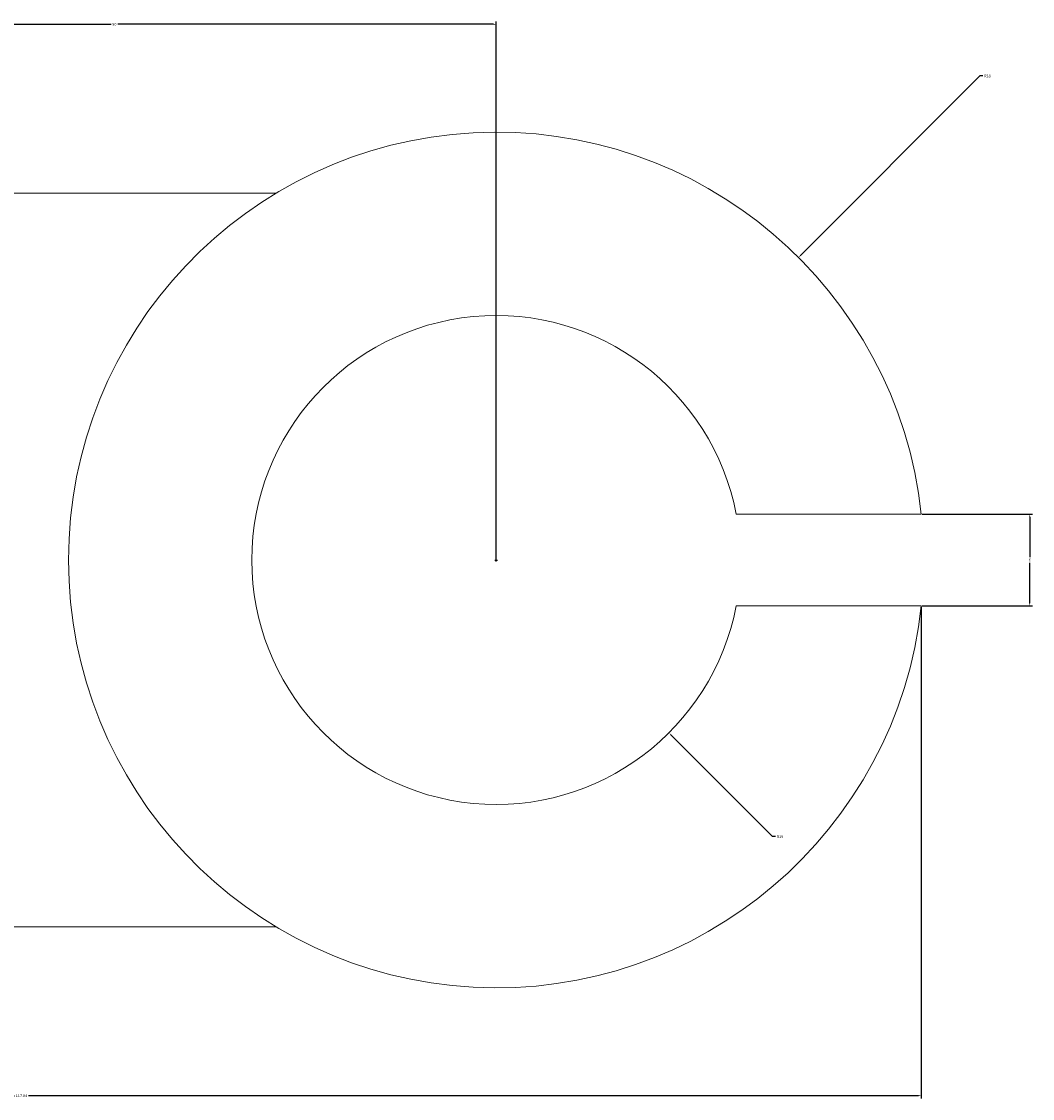
# Model space of a CAD drawing. Units: millimetres. Extents: x 4402 to 4534, y 1655 to 1725.
# Tile 2 of 2: x 4468 to 4534, y 1655 to 1725. Entities that reach past the tile are written whole.
import ezdxf

# ---------------------------------------------------------------- set-up
doc = ezdxf.new("R2010")
doc.units = ezdxf.units.MM
doc.layers.add('M-CONS', color=8, linetype='Continuous', lineweight=18)
doc.layers.add('M-DIMS', color=2, linetype='Continuous', lineweight=18)
doc.styles.get("Standard").update_dxf_attribs({"font": 'arial.ttf'})
doc.dimstyles.get("Standard").update_dxf_attribs({"dimtxt": 0.18, "dimasz": 0.18, "dimexe": 0.18, "dimexo": 0.0625, "dimgap": 0.09, "dimtad": 0, "dimtih": 1, "dimtoh": 1, "dimdec": 4, "dimzin": 0, "dimdsep": 46, "dimtxsty": 'Standard', "dimcen": 0.09, "dimadec": 0, "dimazin": 0, "dimtfac": 1, "dimtdec": 4, "dimtofl": 0, "dimtmove": 0, "dimatfit": 3, "dimfxl": 1, "dimtolj": 1, "dimtzin": 0, "dimarcsym": 0})

# ---------------------------------------------------------------- blocks, each defined once
blk = doc.blocks.new('*D5')
at = {"layer": 'Defpoints', "color": 0, "transparency": 16777216}
for p in [(4526.677, 1686.994), (4408.838, 1665.994), (4526.677, 1654.934)]:
    blk.add_point(p, dxfattribs=at)
at = {"layer": 'M-DIMS', "color": 0, "lineweight": -2, "transparency": 16777216}
for p, q in [((4526.677, 1686.932), (4526.677, 1654.754)), ((4408.838, 1665.932), (4408.838, 1654.754)), ((4409.018, 1654.934), (4467.303, 1654.934)), ((4526.497, 1654.934), (4468.212, 1654.934))]:
    blk.add_line(p, q, dxfattribs=at)
at = {"layer": 'M-DIMS', "color": 0, "transparency": 16777216}
for points in [[(4409.018, 1654.964), (4409.018, 1654.904), (4408.838, 1654.934)], [(4526.497, 1654.964), (4526.497, 1654.904), (4526.677, 1654.934)]]:
    blk.add_solid(points, dxfattribs=at)
at = {"layer": 'M-DIMS', "color": 0, "transparency": 16777216, "insert": (4467.757, 1654.934), "char_height": 0.18, "attachment_point": 5}
blk.add_mtext('\\A1;117.84', dxfattribs=at)
blk = doc.blocks.new('*D6')
at = {"layer": 'Defpoints', "color": 0, "transparency": 16777216}
for p in [(4498.838, 1725.054), (4448.838, 1705.994), (4498.838, 1689.994)]:
    blk.add_point(p, dxfattribs=at)
at = {"layer": 'M-DIMS', "color": 0, "lineweight": -2, "transparency": 16777216}
for p, q in [((4448.838, 1706.057), (4448.838, 1725.234)), ((4449.018, 1725.054), (4473.619, 1725.054)), ((4498.658, 1725.054), (4474.057, 1725.054)), ((4498.838, 1690.057), (4498.838, 1725.234))]:
    blk.add_line(p, q, dxfattribs=at)
at = {"layer": 'M-DIMS', "color": 0, "transparency": 16777216}
for points in [[(4449.018, 1725.084), (4449.018, 1725.024), (4448.838, 1725.054)], [(4498.658, 1725.084), (4498.658, 1725.024), (4498.838, 1725.054)]]:
    blk.add_solid(points, dxfattribs=at)
at = {"layer": 'M-DIMS', "color": 0, "transparency": 16777216, "insert": (4473.838, 1725.054), "char_height": 0.18, "attachment_point": 5}
blk.add_mtext('\\A1;50', dxfattribs=at)
blk = doc.blocks.new('*D7')
at = {"layer": 'Defpoints', "color": 0, "transparency": 16777216}
for p in [(4526.677, 1692.994), (4533.777, 1692.994), (4526.677, 1686.994)]:
    blk.add_point(p, dxfattribs=at)
at = {"layer": 'M-DIMS', "color": 0, "lineweight": -2, "transparency": 16777216}
for p, q in [((4526.739, 1692.994), (4533.957, 1692.994)), ((4533.777, 1692.814), (4533.777, 1690.176)), ((4533.777, 1687.174), (4533.777, 1689.812)), ((4526.739, 1686.994), (4533.957, 1686.994))]:
    blk.add_line(p, q, dxfattribs=at)
at = {"layer": 'M-DIMS', "color": 0, "transparency": 16777216}
for points in [[(4533.747, 1692.814), (4533.807, 1692.814), (4533.777, 1692.994)], [(4533.747, 1687.174), (4533.807, 1687.174), (4533.777, 1686.994)]]:
    blk.add_solid(points, dxfattribs=at)
at = {"layer": 'M-DIMS', "color": 0, "transparency": 16777216, "insert": (4533.777, 1689.994), "char_height": 0.18, "attachment_point": 5}
blk.add_mtext('\\A1;6', dxfattribs=at)
blk = doc.blocks.new('*D8')
at = {"layer": 'Defpoints', "color": 0, "transparency": 16777216}
for p in [(4518.637, 1709.794), (4498.838, 1689.994)]:
    blk.add_point(p, dxfattribs=at)
at = {"layer": 'M-DIMS', "color": 0, "lineweight": -2, "transparency": 16777216}
for p, q in [((4530.516, 1721.673), (4518.764, 1709.921)), ((4530.696, 1721.673), (4530.516, 1721.673)), ((4498.748, 1689.994), (4498.928, 1689.994)), ((4498.838, 1689.904), (4498.838, 1690.084))]:
    blk.add_line(p, q, dxfattribs=at)
at = {"layer": 'M-DIMS', "color": 0, "transparency": 16777216}
blk.add_solid([(4518.743, 1709.942), (4518.785, 1709.9), (4518.637, 1709.794)], dxfattribs=at)
at = {"layer": 'M-DIMS', "color": 0, "transparency": 16777216, "insert": (4531.001, 1721.673), "char_height": 0.18, "attachment_point": 5}
blk.add_mtext('\\A1;R28', dxfattribs=at)
blk = doc.blocks.new('*D9')
at = {"layer": 'Defpoints', "color": 0, "transparency": 16777216}
for p in [(4498.838, 1689.994), (4510.152, 1678.68)]:
    blk.add_point(p, dxfattribs=at)
at = {"layer": 'M-DIMS', "color": 0, "lineweight": -2, "transparency": 16777216}
for p, q in [((4498.748, 1689.994), (4498.928, 1689.994)), ((4498.838, 1689.904), (4498.838, 1690.084)), ((4516.94, 1671.892), (4510.279, 1678.553)), ((4517.12, 1671.892), (4516.94, 1671.892))]:
    blk.add_line(p, q, dxfattribs=at)
at = {"layer": 'M-DIMS', "color": 0, "transparency": 16777216}
blk.add_solid([(4510.3, 1678.574), (4510.258, 1678.532), (4510.152, 1678.68)], dxfattribs=at)
at = {"layer": 'M-DIMS', "color": 0, "transparency": 16777216, "insert": (4517.425, 1671.892), "char_height": 0.18, "attachment_point": 5}
blk.add_mtext('\\A1;R16', dxfattribs=at)

msp = doc.modelspace()

# ---------------------------------------------------------------- linework, layer by layer
at = {"layer": 'M-CONS'}
msp.add_lwpolyline([(4526.677, 1692.994), (4514.554, 1692.994, 10.572078), (4514.554, 1686.994), (4526.677, 1686.994, -18.612941)], format="xyb", close=True, dxfattribs=at)
msp.add_lwpolyline([(4484.416, 1665.994), (4408.838, 1665.994), (4408.838, 1713.994), (4484.416, 1713.994)], dxfattribs=at)

# ---------------------------------------------------------------- dimensions: what is measured, and where the dimension line sits
at = {"layer": 'M-DIMS'}
for base, p1, p2, override, picture, middle in [((4498.838, 1725.054), (4448.838, 1705.994), (4498.838, 1689.994), {"dimdec": 0, "dimlfac": 1, "dimrnd": 0, "dimzin": 0, "dimdsep": 46, "dimlunit": 2}, '*D6', (4473.838, 1725.054)), ((4526.677, 1654.934), (4408.838, 1665.994), (4526.677, 1686.994), {"dimdec": 2, "dimlfac": 1, "dimrnd": 0, "dimzin": 0, "dimdsep": 46, "dimlunit": 2}, '*D5', (4467.757, 1654.934))]:
    dim = msp.add_linear_dim(base=base, p1=p1, p2=p2, dimstyle='Standard', override=override, dxfattribs=at)
    dim.commit()
    dim.dimension.update_dxf_attribs({"geometry": picture, "text_midpoint": middle})
for mpoint, picture, middle in [((4518.637, 1709.794), '*D8', (4531.001, 1721.673)), ((4510.152, 1678.68), '*D9', (4517.425, 1671.892))]:
    dim = msp.add_radius_dim(center=(4498.838, 1689.994), mpoint=mpoint, dimstyle='Standard', override={"dimdec": 0, "dimlfac": 1, "dimrnd": 0, "dimzin": 0, "dimdsep": 46, "dimlunit": 2}, dxfattribs=at)
    dim.commit()
    dim.dimension.update_dxf_attribs({"geometry": picture, "text_midpoint": middle, "dimtype": 164})
dim = msp.add_linear_dim(base=(4533.777, 1692.994), p1=(4526.677, 1686.994), p2=(4526.677, 1692.994), angle=90, dimstyle='Standard', override={"dimdec": 0, "dimlfac": 1, "dimrnd": 0, "dimzin": 0, "dimdsep": 46, "dimlunit": 2}, dxfattribs=at)
dim.commit()
dim.dimension.update_dxf_attribs({"geometry": '*D7', "text_midpoint": (4533.777, 1689.994)})

doc.saveas('drawing.dxf')
